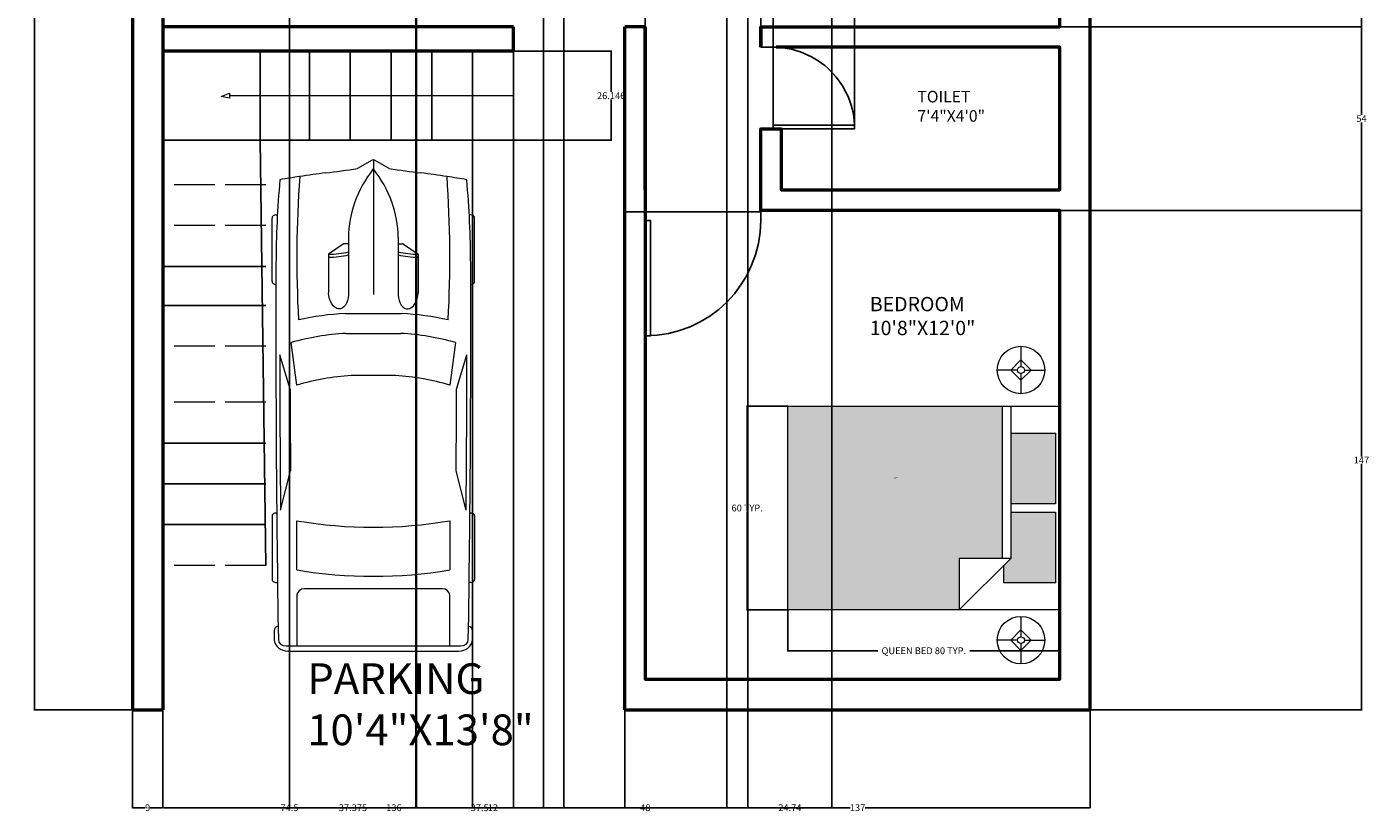
# Model space of a CAD drawing. Units: inches. Extents: x 32 to 429, y 30 to 648.
# Tile 1 of 3: x 32 to 427, y 30 to 261. Entities that reach past the tile are written whole.
import ezdxf

# ---------------------------------------------------------------- set-up
doc = ezdxf.new("R2010")
doc.units = ezdxf.units.IN
doc.header["$MEASUREMENT"] = 0
doc.linetypes.add('ACAD_ISO02W100', pattern=[15, 12, -3])
for name, color, linetype, lineweight in [('A-ANNO-DIMS', 2, 'Continuous', 18), ('A-ANNO-SYMB', 2, 'Continuous', 18), ('A-AREA-IDEN', 7, 'Continuous', 25), ('A-DOOR', 4, 'Continuous', 25), ('A-EQPM-VEHL', 8, 'Continuous', 18), ('A-FLOR-STRS', 7, 'Continuous', 25), ('A-FLOR-STRS-HIDN', 8, 'ACAD_ISO02W100', 18), ('A-FURN', 9, 'Continuous', 18), ('A-FURN-PATT', 252, 'Continuous', 13), ('A-WALL', 7, 'Continuous', 50)]:
    doc.layers.add(name, color=color, linetype=linetype, lineweight=lineweight)
doc.styles.get("Standard").update_dxf_attribs({"font": 'arial.ttf'})
doc.dimstyles.get("Standard").update_dxf_attribs({"dimtxt": 2, "dimasz": 0.18, "dimexe": 0.18, "dimexo": 0.0625, "dimgap": 0.09, "dimtad": 0, "dimtih": 1, "dimtoh": 1, "dimrnd": 2, "dimzin": 0, "dimdsep": 46, "dimlunit": 3, "dimtxsty": 'Standard', "dimcen": 0.09, "dimadec": 0, "dimazin": 0, "dimtfac": 1, "dimtofl": 0, "dimtmove": 0, "dimatfit": 3, "dimfxl": 1, "dimtolj": 1, "dimtzin": 0, "dimarcsym": 0})
pattern_1 = [(0, (0, -434.5), (0.03125, 0.0625), [0, -0.0625])]

# ---------------------------------------------------------------- blocks, each defined once
blk = doc.blocks.new('*U5')
for p, q in [((21.1, 37.41), (21.1, 36.83)), ((46.55, 38.89), (22.35, 38.89)), ((47.8, 37.39), (47.8, 37.41)), ((135.45, 37.07), (135.45, 37.41)), ((136.7, 38.89), (160.9, 38.89)), ((162.15, 37.41), (162.15, 36.77)), ((70.03, 31.54), (86.41, 29.35)), ((87.99, 31.87), (74.76, 35.92)), ((134.31, 35.6), (119.29, 31.78)), ((186.47, -33.5), (186.47, 33.5)), ((188.4, -32.76), (188.4, 32.76)), ((138.42, 29.35), (157.25, 29.35)), ((164.52, 26.39), (164.52, -26.39)), ((186.47, 29.35), (167.01, 29.35)), ((32.27, 11.63), (36.13, 17.17)), ((36.13, 17.17), (50.94, 17.17)), ((32.12, 9.51), (32.12, 11.15)), ((58.92, -10.77), (58.92, 10.77)), ((66.55, -10.53), (66.55, 10.53)), ((186.47, -10.53), (186.47, 10.53)), ((3.27, 6.13), (0.1, 0.41)), ((29.77, 9.51), (51.68, 9.51)), ((82.74, 8.5), (82.74, -8.5)), ((0, 0), (51.68, 0)), ((0.1, -0.41), (3.27, -6.13)), ((29.77, -9.51), (51.68, -9.51)), ((32.12, -9.51), (32.12, -11.15)), ((32.27, -11.63), (36.13, -17.17)), ((36.13, -17.17), (50.94, -17.17)), ((86.41, -29.35), (70.03, -31.54)), ((157.25, -29.35), (138.42, -29.35)), ((167.01, -29.35), (186.47, -29.35)), ((87.99, -31.87), (74.76, -35.92)), ((134.31, -35.6), (119.29, -31.78)), ((21.1, -37.41), (21.1, -36.83)), ((46.55, -38.89), (22.35, -38.89)), ((47.8, -37.39), (47.8, -37.41)), ((135.45, -37.07), (135.45, -37.41)), ((136.7, -38.89), (160.9, -38.89)), ((162.15, -37.41), (162.15, -36.77))]:
    blk.add_line(p, q)
for centre, major_axis, ratio, start_param, end_param in [((41.19, -490.86), (0, 528.23), 0.842304, 0.00281, 0.075598), ((22.35, 37.41), (0, -1.48), 0.842304, 3.141593, 4.712389), ((64.48, -10555.62), (0, 10593.03), 0.842304, -0.013397, 0.002797), ((46.55, 37.41), (0, 1.48), 0.842304, -1.570796, 0), ((136.7, 37.41), (0, -1.48), 0.842304, 3.141593, 4.712389), ((160.9, 37.41), (0, 1.48), 0.842304, -1.570796, 0), ((180.63, 35.84), (0, 2.22), 0.842304, -0.013017, 1.249894), ((64.48, -10556.36), (0, 10595.31), 0.842304, -0.013397, -0.013017), ((183.98, 33.5), (0, -2.96), 0.842304, 1.570796, 3.128196), ((183.98, 32.76), (0, -5.25), 0.842304, 1.570796, 3.128196), ((266.03, -27.52), (0, 313.31), 0.842304, 1.367076, 1.39176), ((135.29, 5.39), (0, 81.77), 0.842304, 1.245306, 1.50788), ((64.48, -10555.62), (0, -10591.55), 0.842304, 3.133765, 3.140441), ((95.79, -3666.35), (0, -3698.24), 0.842304, 3.134049, 3.144098), ((259.18, -27.52), (0, -305.3), 0.842304, 4.528606, 4.561838), ((37.47, -593.96), (0, -623.33), 0.842304, 3.096046, 3.200911), ((134.4, 5.39), (0, -89.78), 0.842304, 4.449482, 4.652344), ((149.6, 2.8), (0, -79.58), 0.842304, 4.372215, 4.640744), ((17.08, 0), (0, 147.02), 0.842304, 4.511394, 4.913384), ((35.91, 0), (0, 147.02), 0.842304, 4.511394, 4.913384), ((167.01, 26.39), (0, 2.96), 0.842304, 0, 1.570796), ((-204.49, 52.4), (0, -250.96), 0.842304, 1.385369, 1.434372), ((13.04, 17.01), (0, 27.42), 0.842304, 4.435146, 4.718221), ((14.2, 17.01), (0, 27.42), 0.842304, 4.435146, 4.718221), ((50.79, 13.34), (6.34, -0.36), 0.603834, -1.395552, 1.581315), ((32.75, 11.15), (0, 0.74), 0.842304, 0.879714, 1.570796), ((29.77, -46.66), (0, 56.17), 0.842304, 0, 0.590319), ((0.62, 0), (0, -0.74), 0.842304, 4.131459, 5.293319), ((29.77, 46.66), (0, 56.17), 0.842304, 2.551274, 3.141593), ((-204.49, -52.4), (0, 250.96), 0.842304, -1.434372, -1.385369), ((13.04, -17.01), (0, -27.42), 0.842304, 1.564964, 1.848039), ((14.2, -17.01), (0, -27.42), 0.842304, 1.564964, 1.848039), ((149.6, -2.8), (0, -79.58), 0.842304, -1.499151, -1.230623), ((32.75, -11.15), (0, -0.74), 0.842304, 4.712389, 5.403472), ((134.4, -5.39), (0, -89.78), 0.842304, -1.510751, -1.307889), ((135.29, -5.39), (0, -81.77), 0.842304, -1.50788, -1.245306), ((259.18, 27.52), (0, 305.3), 0.842304, 1.721348, 1.754579), ((266.03, 27.52), (0, 313.31), 0.842304, 1.749832, 1.774517), ((37.47, 593.96), (0, -623.33), 0.842304, -0.059319, 0.045547), ((167.01, -26.39), (0, -2.96), 0.842304, 4.712389, 6.283185), ((41.19, 490.86), (0, -528.23), 0.842304, -0.075598, -0.00281), ((64.48, 10555.62), (0, -10591.55), 0.842304, 0.001152, 0.007828), ((95.79, 3666.35), (0, -3698.24), 0.842304, -0.002505, 0.007544), ((183.98, -33.5), (0, 2.96), 0.842304, 3.15499, 4.712389), ((183.98, -32.76), (0, -5.25), 0.842304, 0.013397, 1.570796), ((22.35, -37.41), (0, 1.48), 0.842304, 1.570796, 3.141593), ((64.48, 10555.62), (0, 10593.03), 0.842304, 3.138796, 3.15499), ((46.55, -37.41), (0, -1.48), 0.842304, 0, 1.570796), ((136.7, -37.41), (0, -1.48), 0.842304, -1.570796, 0), ((160.9, -37.41), (0, 1.48), 0.842304, 3.141593, 4.712389), ((180.63, -35.84), (0, -2.22), 0.842304, -1.249894, 0.013017), ((64.48, 10556.36), (0, 10595.31), 0.842304, 3.15461, 3.15499)]:
    blk.add_ellipse(centre, major_axis=major_axis, ratio=ratio, start_param=start_param, end_param=end_param)
at = {"extrusion": (0, 0, -1)}
blk.add_ellipse((50.79, -13.34), major_axis=(6.34, 0.36), ratio=0.603834, start_param=-1.395552, end_param=1.581315, dxfattribs=at)
blk = doc.blocks.new('*U7')
for p, q in [((0, 0), (0, 6)), ((40, 0), (40, 6))]:
    blk.add_line(p, q)
blk.add_lwpolyline([(0, 0), (0, -40), (1.75, -40), (1.75, 0)], close=True)
blk.add_arc((0, 0), 40, 270, 0)
blk = doc.blocks.new('Bed - Queen')
for p, q in [((0, -80.00003), (0, 0)), ((0, 0), (59.99999, 0)), ((59.99999, 0), (59.99999, -80.00003)), ((7.99999, -1.2), (28.79998, -1.2)), ((7.99999, -14.4), (7.99999, -1.2)), ((28.79998, -1.2), (28.79998, -14.4)), ((31.19999, -1.2), (51.99999, -1.2)), ((31.19999, -14.4), (31.19999, -1.2)), ((51.99999, -1.2), (51.99999, -16.4)), ((0, -14.4), (44.8, -14.4)), ((59.99999, -29.6), (44.8, -14.4)), ((44.8, -14.4), (44.8, -29.6)), ((44.8, -16.8), (0, -16.8)), ((51.99999, -16.4), (46.79936, -16.4)), ((44.8, -29.6), (59.99999, -29.6)), ((59.99999, -80.00003), (0, -80.00003))]:
    blk.add_line(p, q)
blk = doc.blocks.new('Lamp - Table')
for p, q in [((0, 7), (0, 1)), ((-1, 0), (-7, 0)), ((0, 3), (-3, 0)), ((-3, 0), (0, -3)), ((3, 0), (0, 3)), ((0, -3), (3, 0)), ((1, 0), (7, 0)), ((0, -1), (0, -7))]:
    blk.add_line(p, q)
for radius in [7, 1]:
    blk.add_circle((0, 0), radius)
blk = doc.blocks.new('*D17')
at = {"layer": 'A-ANNO-DIMS', "color": 0, "lineweight": -2, "transparency": 16777216}
for p, q in [((256.39, 89.31), (256.39, 77.2)), ((336.39, 89.31), (336.39, 77.2)), ((256.57, 77.38), (282.82, 77.38)), ((336.21, 77.38), (309.97, 77.38))]:
    blk.add_line(p, q, dxfattribs=at)
at = {"layer": 'A-ANNO-DIMS', "color": 0, "transparency": 16777216}
for points in [[(256.57, 77.41), (256.57, 77.35), (256.39, 77.38)], [(336.21, 77.41), (336.21, 77.35), (336.39, 77.38)]]:
    blk.add_solid(points, dxfattribs=at)
at = {"layer": 'Defpoints', "color": 0, "transparency": 16777216}
for p in [(256.39, 89.38), (336.39, 89.38), (336.39, 77.38)]:
    blk.add_point(p, dxfattribs=at)
at = {"layer": 'A-ANNO-DIMS', "color": 0, "transparency": 16777216, "insert": (296.39, 77.38), "char_height": 2, "attachment_point": 5}
blk.add_mtext('\\A1;QUEEN BED 80 TYP.', dxfattribs=at)
blk = doc.blocks.new('*D18')
at = {"layer": 'A-ANNO-DIMS', "color": 0, "lineweight": -2, "transparency": 16777216}
for p, q in [((256.33, 149.38), (244.21, 149.38)), ((244.39, 149.2), (244.39, 120.49)), ((244.39, 89.56), (244.39, 118.27)), ((256.33, 89.38), (244.21, 89.38))]:
    blk.add_line(p, q, dxfattribs=at)
at = {"layer": 'A-ANNO-DIMS', "color": 0, "transparency": 16777216}
for points in [[(244.36, 149.2), (244.42, 149.2), (244.39, 149.38)], [(244.36, 89.56), (244.42, 89.56), (244.39, 89.38)]]:
    blk.add_solid(points, dxfattribs=at)
at = {"layer": 'Defpoints', "color": 0, "transparency": 16777216}
for p in [(256.39, 149.38), (244.39, 89.38), (256.39, 89.38)]:
    blk.add_point(p, dxfattribs=at)
at = {"layer": 'A-ANNO-DIMS', "color": 0, "transparency": 16777216, "insert": (244.39, 119.38), "char_height": 2, "attachment_point": 5}
blk.add_mtext('\\A1;60 TYP.', dxfattribs=at)
blk = doc.blocks.new('*D34')
at = {"layer": 'A-ANNO-DIMS', "color": 0, "lineweight": -2, "transparency": 16777216}
for p, q in [((63.33, 617.99), (34.41, 617.99)), ((34.59, 617.81), (34.59, 340.1)), ((34.59, 60.17), (34.59, 337.88)), ((63.33, 59.99), (34.41, 59.99))]:
    blk.add_line(p, q, dxfattribs=at)
at = {"layer": 'A-ANNO-DIMS', "color": 0, "transparency": 16777216}
for points in [[(34.56, 617.81), (34.62, 617.81), (34.59, 617.99)], [(34.56, 60.17), (34.62, 60.17), (34.59, 59.99)]]:
    blk.add_solid(points, dxfattribs=at)
at = {"layer": 'Defpoints', "color": 0, "transparency": 16777216}
for p in [(34.59, 617.99), (63.39, 617.99), (63.39, 59.99)]:
    blk.add_point(p, dxfattribs=at)
at = {"layer": 'A-ANNO-DIMS', "color": 0, "transparency": 16777216, "insert": (34.59, 338.99), "char_height": 2, "attachment_point": 5}
blk.add_mtext('\\A1;558', dxfattribs=at)
blk = doc.blocks.new('*D35')
at = {"layer": 'A-ANNO-DIMS', "color": 0, "lineweight": -2, "transparency": 16777216}
for p, q in [((63.39, 59.93), (63.39, 31.01)), ((72.39, 59.93), (72.39, 31.01)), ((63.57, 31.19), (67.15, 31.19)), ((72.21, 31.19), (68.64, 31.19))]:
    blk.add_line(p, q, dxfattribs=at)
at = {"layer": 'A-ANNO-DIMS', "color": 0, "transparency": 16777216}
for points in [[(63.57, 31.22), (63.57, 31.16), (63.39, 31.19)], [(72.21, 31.22), (72.21, 31.16), (72.39, 31.19)]]:
    blk.add_solid(points, dxfattribs=at)
at = {"layer": 'Defpoints', "color": 0, "transparency": 16777216}
for p in [(63.39, 59.99), (72.39, 59.99), (72.39, 31.19)]:
    blk.add_point(p, dxfattribs=at)
at = {"layer": 'A-ANNO-DIMS', "color": 0, "transparency": 16777216, "insert": (67.89, 31.19), "char_height": 2, "attachment_point": 5}
blk.add_mtext('\\A1;9', dxfattribs=at)
blk = doc.blocks.new('*D36')
at = {"layer": 'A-ANNO-DIMS', "color": 0, "lineweight": -2, "transparency": 16777216}
for p, q in [((72.39, 59.93), (72.39, 31.01)), ((208.39, 59.93), (208.39, 31.01)), ((72.57, 31.19), (138.19, 31.19)), ((208.21, 31.19), (142.6, 31.19))]:
    blk.add_line(p, q, dxfattribs=at)
at = {"layer": 'A-ANNO-DIMS', "color": 0, "transparency": 16777216}
for points in [[(72.57, 31.22), (72.57, 31.16), (72.39, 31.19)], [(208.21, 31.22), (208.21, 31.16), (208.39, 31.19)]]:
    blk.add_solid(points, dxfattribs=at)
at = {"layer": 'Defpoints', "color": 0, "transparency": 16777216}
for p in [(72.39, 59.99), (208.39, 59.99), (208.39, 31.19)]:
    blk.add_point(p, dxfattribs=at)
at = {"layer": 'A-ANNO-DIMS', "color": 0, "transparency": 16777216, "insert": (140.39, 31.19), "char_height": 2, "attachment_point": 5}
blk.add_mtext('\\A1;136', dxfattribs=at)
blk = doc.blocks.new('*D37')
at = {"layer": 'A-ANNO-DIMS', "color": 0, "lineweight": -2, "transparency": 16777216}
for p, q in [((208.39, 59.93), (208.39, 31.01)), ((345.39, 59.93), (345.39, 31.01)), ((208.57, 31.19), (274.69, 31.19)), ((345.21, 31.19), (279.1, 31.19))]:
    blk.add_line(p, q, dxfattribs=at)
at = {"layer": 'A-ANNO-DIMS', "color": 0, "transparency": 16777216}
for points in [[(208.57, 31.22), (208.57, 31.16), (208.39, 31.19)], [(345.21, 31.22), (345.21, 31.16), (345.39, 31.19)]]:
    blk.add_solid(points, dxfattribs=at)
at = {"layer": 'Defpoints', "color": 0, "transparency": 16777216}
for p in [(208.39, 59.99), (345.39, 59.99), (345.39, 31.19)]:
    blk.add_point(p, dxfattribs=at)
at = {"layer": 'A-ANNO-DIMS', "color": 0, "transparency": 16777216, "insert": (276.89, 31.19), "char_height": 2, "attachment_point": 5}
blk.add_mtext('\\A1;137', dxfattribs=at)
blk = doc.blocks.new('*D38')
at = {"layer": 'A-ANNO-DIMS', "color": 0, "lineweight": -2, "transparency": 16777216}
for p, q in [((336.46, 206.99), (425.41, 206.99)), ((425.23, 206.81), (425.23, 134.59)), ((425.23, 60.17), (425.23, 132.4)), ((345.46, 59.99), (425.41, 59.99))]:
    blk.add_line(p, q, dxfattribs=at)
at = {"layer": 'A-ANNO-DIMS', "color": 0, "transparency": 16777216}
for points in [[(425.2, 206.81), (425.26, 206.81), (425.23, 206.99)], [(425.2, 60.17), (425.26, 60.17), (425.23, 59.99)]]:
    blk.add_solid(points, dxfattribs=at)
at = {"layer": 'Defpoints', "color": 0, "transparency": 16777216}
for p in [(336.39, 206.99), (425.23, 206.99), (345.39, 59.99)]:
    blk.add_point(p, dxfattribs=at)
at = {"layer": 'A-ANNO-DIMS', "color": 0, "transparency": 16777216, "insert": (425.23, 133.49), "char_height": 2, "attachment_point": 5}
blk.add_mtext('\\A1;147', dxfattribs=at)
blk = doc.blocks.new('*D39')
at = {"layer": 'A-ANNO-DIMS', "color": 0, "lineweight": -2, "transparency": 16777216}
for p, q in [((336.46, 260.99), (425.41, 260.99)), ((425.23, 260.81), (425.23, 235.1)), ((425.23, 207.17), (425.23, 232.89)), ((336.46, 206.99), (425.41, 206.99))]:
    blk.add_line(p, q, dxfattribs=at)
at = {"layer": 'A-ANNO-DIMS', "color": 0, "transparency": 16777216}
for points in [[(425.2, 260.81), (425.26, 260.81), (425.23, 260.99)], [(425.2, 207.17), (425.26, 207.17), (425.23, 206.99)]]:
    blk.add_solid(points, dxfattribs=at)
at = {"layer": 'Defpoints', "color": 0, "transparency": 16777216}
for p in [(336.39, 260.99), (425.23, 260.99), (336.39, 206.99)]:
    blk.add_point(p, dxfattribs=at)
at = {"layer": 'A-ANNO-DIMS', "color": 0, "transparency": 16777216, "insert": (425.23, 233.99), "char_height": 2, "attachment_point": 5}
blk.add_mtext('\\A1;54', dxfattribs=at)
blk = doc.blocks.new('*D40')
at = {"layer": 'A-ANNO-DIMS', "color": 0, "lineweight": -2, "transparency": 16777216}
for p, q in [((336.46, 426.99), (425.41, 426.99)), ((425.23, 426.81), (425.23, 345.1)), ((425.23, 261.17), (425.23, 342.88)), ((336.46, 260.99), (425.41, 260.99))]:
    blk.add_line(p, q, dxfattribs=at)
at = {"layer": 'A-ANNO-DIMS', "color": 0, "transparency": 16777216}
for points in [[(425.2, 426.81), (425.26, 426.81), (425.23, 426.99)], [(425.2, 261.17), (425.26, 261.17), (425.23, 260.99)]]:
    blk.add_solid(points, dxfattribs=at)
at = {"layer": 'Defpoints', "color": 0, "transparency": 16777216}
for p in [(336.39, 426.99), (425.23, 426.99), (336.39, 260.99)]:
    blk.add_point(p, dxfattribs=at)
at = {"layer": 'A-ANNO-DIMS', "color": 0, "transparency": 16777216, "insert": (425.23, 343.99), "char_height": 2, "attachment_point": 5}
blk.add_mtext('\\A1;166', dxfattribs=at)
blk = doc.blocks.new('*D43')
at = {"layer": 'A-ANNO-DIMS', "color": 0, "lineweight": -2, "transparency": 16777216}
for p, q in [((72.39, 426.93), (72.39, 31.01)), ((146.89, 426.93), (146.89, 31.01)), ((72.57, 31.19), (106.96, 31.19)), ((146.71, 31.19), (112.33, 31.19))]:
    blk.add_line(p, q, dxfattribs=at)
at = {"layer": 'A-ANNO-DIMS', "color": 0, "transparency": 16777216}
for points in [[(72.57, 31.22), (72.57, 31.16), (72.39, 31.19)], [(146.71, 31.22), (146.71, 31.16), (146.89, 31.19)]]:
    blk.add_solid(points, dxfattribs=at)
at = {"layer": 'Defpoints', "color": 0, "transparency": 16777216}
for p in [(72.39, 426.99), (146.89, 426.99), (146.89, 31.19)]:
    blk.add_point(p, dxfattribs=at)
at = {"layer": 'A-ANNO-DIMS', "color": 0, "transparency": 16777216, "insert": (109.64, 31.19), "char_height": 2, "attachment_point": 5}
blk.add_mtext('\\A1;74.5', dxfattribs=at)
blk = doc.blocks.new('*D44')
at = {"layer": 'A-ANNO-DIMS', "color": 0, "lineweight": -2, "transparency": 16777216}
for p, q in [((146.89, 426.93), (146.89, 31.01)), ((184.39, 426.93), (184.39, 31.01)), ((147.07, 31.19), (162.95, 31.19)), ((184.21, 31.19), (168.34, 31.19))]:
    blk.add_line(p, q, dxfattribs=at)
at = {"layer": 'A-ANNO-DIMS', "color": 0, "transparency": 16777216}
for points in [[(147.07, 31.22), (147.07, 31.16), (146.89, 31.19)], [(184.21, 31.22), (184.21, 31.16), (184.39, 31.19)]]:
    blk.add_solid(points, dxfattribs=at)
at = {"layer": 'Defpoints', "color": 0, "transparency": 16777216}
for p in [(146.89, 426.99), (184.39, 426.99), (184.39, 31.19)]:
    blk.add_point(p, dxfattribs=at)
at = {"layer": 'A-ANNO-DIMS', "color": 0, "transparency": 16777216, "insert": (165.64, 31.19), "char_height": 2, "attachment_point": 5}
blk.add_mtext('\\A1;37.5', dxfattribs=at)
blk = doc.blocks.new('*D45')
at = {"layer": 'A-ANNO-DIMS', "color": 0, "lineweight": -2, "transparency": 16777216}
for p, q in [((190.39, 426.93), (190.39, 31.01)), ((238.39, 426.93), (238.39, 31.01)), ((190.57, 31.19), (212.83, 31.19)), ((238.21, 31.19), (215.96, 31.19))]:
    blk.add_line(p, q, dxfattribs=at)
at = {"layer": 'A-ANNO-DIMS', "color": 0, "transparency": 16777216}
for points in [[(190.57, 31.22), (190.57, 31.16), (190.39, 31.19)], [(238.21, 31.22), (238.21, 31.16), (238.39, 31.19)]]:
    blk.add_solid(points, dxfattribs=at)
at = {"layer": 'Defpoints', "color": 0, "transparency": 16777216}
for p in [(190.39, 426.99), (238.39, 426.99), (238.39, 31.19)]:
    blk.add_point(p, dxfattribs=at)
at = {"layer": 'A-ANNO-DIMS', "color": 0, "transparency": 16777216, "insert": (214.39, 31.19), "char_height": 2, "attachment_point": 5}
blk.add_mtext('\\A1;48', dxfattribs=at)
blk = doc.blocks.new('*D47')
at = {"layer": 'A-ANNO-DIMS', "color": 0, "lineweight": -2, "transparency": 16777216}
for p, q in [((214.39, 261.06), (214.39, 646.97)), ((214.57, 646.79), (229.88, 646.79)), ((248.21, 646.79), (232.91, 646.79)), ((248.39, 261.06), (248.39, 646.97))]:
    blk.add_line(p, q, dxfattribs=at)
at = {"layer": 'A-ANNO-DIMS', "color": 0, "transparency": 16777216}
for points in [[(214.57, 646.82), (214.57, 646.76), (214.39, 646.79)], [(248.21, 646.82), (248.21, 646.76), (248.39, 646.79)]]:
    blk.add_solid(points, dxfattribs=at)
at = {"layer": 'Defpoints', "color": 0, "transparency": 16777216}
for p in [(248.39, 646.79), (214.39, 260.99), (248.39, 260.99)]:
    blk.add_point(p, dxfattribs=at)
at = {"layer": 'A-ANNO-DIMS', "color": 0, "transparency": 16777216, "insert": (231.39, 646.79), "char_height": 2, "attachment_point": 5}
blk.add_mtext('\\A1;34', dxfattribs=at)
blk = doc.blocks.new('*D49')
at = {"layer": 'A-ANNO-DIMS', "color": 0, "lineweight": -2, "transparency": 16777216}
for p, q in [((109.64, 529.9), (109.64, 31.01)), ((147.02, 529.9), (147.02, 31.01)), ((109.82, 31.19), (124.08, 31.19)), ((146.84, 31.19), (132.58, 31.19))]:
    blk.add_line(p, q, dxfattribs=at)
at = {"layer": 'A-ANNO-DIMS', "color": 0, "transparency": 16777216}
for points in [[(109.82, 31.22), (109.82, 31.16), (109.64, 31.19)], [(146.84, 31.22), (146.84, 31.16), (147.02, 31.19)]]:
    blk.add_solid(points, dxfattribs=at)
at = {"layer": 'Defpoints', "color": 0, "transparency": 16777216}
for p in [(109.64, 529.96), (147.02, 529.96), (147.02, 31.19)]:
    blk.add_point(p, dxfattribs=at)
at = {"layer": 'A-ANNO-DIMS', "color": 0, "transparency": 16777216, "insert": (128.33, 31.19), "char_height": 2, "attachment_point": 5}
blk.add_mtext('\\A1;37.375', dxfattribs=at)
blk = doc.blocks.new('*D51')
at = {"layer": 'A-ANNO-DIMS', "color": 0, "lineweight": -2, "transparency": 16777216}
for p, q in [((244.58, 478.88), (244.58, 31.01)), ((269.32, 478.88), (269.32, 31.01)), ((244.76, 31.19), (253.47, 31.19)), ((269.14, 31.19), (260.43, 31.19))]:
    blk.add_line(p, q, dxfattribs=at)
at = {"layer": 'A-ANNO-DIMS', "color": 0, "transparency": 16777216}
for points in [[(244.76, 31.22), (244.76, 31.16), (244.58, 31.19)], [(269.14, 31.22), (269.14, 31.16), (269.32, 31.19)]]:
    blk.add_solid(points, dxfattribs=at)
at = {"layer": 'Defpoints', "color": 0, "transparency": 16777216}
for p in [(244.58, 478.95), (269.32, 478.95), (269.32, 31.19)]:
    blk.add_point(p, dxfattribs=at)
at = {"layer": 'A-ANNO-DIMS', "color": 0, "transparency": 16777216, "insert": (256.95, 31.19), "char_height": 2, "attachment_point": 5}
blk.add_mtext('\\A1;24.74', dxfattribs=at)
blk = doc.blocks.new('*D52')
at = {"layer": 'A-ANNO-DIMS', "color": 0, "lineweight": -2, "transparency": 16777216}
for p, q in [((252, 232.11), (252, 646.97)), ((252.18, 646.79), (260.54, 646.79)), ((275.84, 646.79), (267.48, 646.79)), ((276.02, 232.11), (276.02, 646.97))]:
    blk.add_line(p, q, dxfattribs=at)
at = {"layer": 'A-ANNO-DIMS', "color": 0, "transparency": 16777216}
for points in [[(252.18, 646.82), (252.18, 646.76), (252, 646.79)], [(275.84, 646.82), (275.84, 646.76), (276.02, 646.79)]]:
    blk.add_solid(points, dxfattribs=at)
at = {"layer": 'Defpoints', "color": 0, "transparency": 16777216}
for p in [(276.02, 646.79), (252, 232.04), (276.02, 232.04)]:
    blk.add_point(p, dxfattribs=at)
at = {"layer": 'A-ANNO-DIMS', "color": 0, "transparency": 16777216, "insert": (264.01, 646.79), "char_height": 2, "attachment_point": 5}
blk.add_mtext('\\A1;24.02', dxfattribs=at)
blk = doc.blocks.new('*D54')
at = {"layer": 'A-ANNO-DIMS', "color": 0, "lineweight": -2, "transparency": 16777216}
for p, q in [((163.55, 227.58), (163.55, 31.01)), ((175.55, 227.58), (175.55, 31.01)), ((163.73, 31.19), (168.13, 31.19)), ((175.37, 31.19), (170.96, 31.19))]:
    blk.add_line(p, q, dxfattribs=at)
at = {"layer": 'A-ANNO-DIMS', "color": 0, "transparency": 16777216}
for points in [[(163.73, 31.22), (163.73, 31.16), (163.55, 31.19)], [(175.37, 31.22), (175.37, 31.16), (175.55, 31.19)]]:
    blk.add_solid(points, dxfattribs=at)
at = {"layer": 'Defpoints', "color": 0, "transparency": 16777216}
for p in [(163.55, 227.65), (175.55, 227.65), (175.55, 31.19)]:
    blk.add_point(p, dxfattribs=at)
at = {"layer": 'A-ANNO-DIMS', "color": 0, "transparency": 16777216, "insert": (169.55, 31.19), "char_height": 2, "attachment_point": 5}
blk.add_mtext('\\A1;12', dxfattribs=at)
blk = doc.blocks.new('*D57')
at = {"layer": 'A-ANNO-DIMS', "color": 0, "lineweight": -2, "transparency": 16777216}
for p, q in [((175.61, 253.79), (204.53, 253.79)), ((204.35, 253.61), (204.35, 241.83)), ((204.35, 227.83), (204.35, 239.61)), ((175.61, 227.65), (204.53, 227.65))]:
    blk.add_line(p, q, dxfattribs=at)
at = {"layer": 'A-ANNO-DIMS', "color": 0, "transparency": 16777216}
for points in [[(204.32, 253.61), (204.38, 253.61), (204.35, 253.79)], [(204.32, 227.83), (204.38, 227.83), (204.35, 227.65)]]:
    blk.add_solid(points, dxfattribs=at)
at = {"layer": 'Defpoints', "color": 0, "transparency": 16777216}
for p in [(175.55, 253.79), (175.55, 227.65), (204.35, 227.65)]:
    blk.add_point(p, dxfattribs=at)
at = {"layer": 'A-ANNO-DIMS', "color": 0, "transparency": 16777216, "insert": (204.35, 240.72), "char_height": 2, "attachment_point": 5}
blk.add_mtext('\\A1;26.146', dxfattribs=at)

msp = doc.modelspace()

# ---------------------------------------------------------------- hatches: boundary and pattern name
at = {"layer": 'A-FURN-PATT'}
h = msp.add_hatch(dxfattribs=at)
h.set_pattern_fill('DOTS', color=256)
h.set_pattern_definition(pattern_1)
h.paths.add_polyline_path([(335.194, 141.3763), (321.994, 141.3763), (321.994, 120.5763), (335.194, 120.5763)])
h.paths.add_polyline_path([(335.194, 118.1763), (321.994, 118.1763), (321.994, 104.5763), (319.994, 102.5763), (319.994, 97.3763), (335.194, 97.3763)])
h.paths.add_polyline_path([(319.594, 149.3763), (256.3939, 149.3763), (256.3939, 89.3763), (306.794, 89.3763), (306.794, 104.5763), (319.594, 104.5763)])
h = msp.add_hatch(dxfattribs=at)
h.set_pattern_fill('DOTS', color=256)
h.set_pattern_definition(pattern_1)
h.paths.add_polyline_path([(319.594, 149.3763), (256.3939, 149.3763), (256.3939, 89.3763), (306.794, 89.3763), (306.794, 104.5763), (319.594, 104.5763)])

# ---------------------------------------------------------------- linework, layer by layer
at = {"layer": 'A-ANNO-SYMB'}
for p, q in [((89.5, 240.5), (92, 241.5)), ((92, 241.5), (92, 240.7197)), ((92, 240), (89.5, 240.5)), ((92, 241), (92, 241)), ((175.5464, 240.7197), (92, 240.7197)), ((92, 240.7197), (92, 240))]:
    msp.add_line(p, q, dxfattribs=at)
at = {"layer": 'A-DOOR'}
msp.add_line((248.3706, 206.589), (208.3942, 206.589), dxfattribs=at)
at = {"layer": 'A-FLOR-STRS'}
for p, q in [((115.5464, 253.7929), (115.5464, 227.6465)), ((127.5464, 253.7929), (127.5464, 227.6465)), ((139.5464, 253.7929), (139.5464, 227.6465)), ((151.5464, 253.7929), (151.5464, 227.6465)), ((163.5464, 253.7929), (163.5464, 227.6465)), ((175.5464, 253.7929), (175.5464, 227.6465)), ((175.5464, 227.6465), (72.3942, 227.6465)), ((101, 227.6465), (102.6949, 102.5)), ((102.6949, 190.5), (72.3942, 190.5)), ((102.6949, 179), (72.3942, 179)), ((102.6949, 179), (72.3942, 179)), ((102.6949, 138.5), (72.3942, 138.5)), ((102.6949, 126.5), (72.3942, 126.5)), ((102.6949, 114.5), (72.3942, 114.5))]:
    msp.add_line(p, q, dxfattribs=at)
msp.add_lwpolyline([(72.3942, 219.5), (72.3942, 253.7929), (101, 253.7929), (101, 227.6465)], dxfattribs=at)
at = {"layer": 'A-FLOR-STRS-HIDN'}
for p, q in [((102.6949, 214.5), (72.3942, 214.5)), ((102.6949, 202.5), (72.3942, 202.5)), ((102.6949, 190.5), (72.3942, 190.5)), ((102.6949, 179), (72.3942, 179)), ((102.6949, 167), (72.3942, 167)), ((102.6949, 150.5), (72.3942, 150.5)), ((102.6949, 138.5), (72.3942, 138.5)), ((102.6949, 126.5), (72.3942, 126.5)), ((102.6949, 114.5), (72.3942, 114.5)), ((102.6949, 102.5), (72.3942, 102.5))]:
    msp.add_line(p, q, dxfattribs=at)
at = {"layer": 'A-WALL'}
for p, q in [((175.5464, 260.9929), (72.3942, 260.9929)), ((175.5464, 253.7929), (175.5464, 260.9929)), ((214.3942, 260.9929), (208.3942, 260.9929)), ((208.3942, 212.9929), (208.3942, 260.9929)), ((214.3942, 212.9929), (214.3942, 260.9929)), ((248.3942, 260.9929), (248.3942, 254.9929)), ((175.5464, 253.7929), (72.3942, 253.7929))]:
    msp.add_line(p, q, dxfattribs=at)
for points in [[(208.3942, 59.9929), (345.3942, 59.9929), (345.3942, 617.9929), (63.3942, 617.9929), (63.3942, 59.9929)], [(248.394, 254.9928), (248.394, 260.9928), (336.394, 260.9928), (336.394, 608.9928), (72.394, 608.9928), (72.394, 59.9928)], [(208.3942, 59.9929), (208.3942, 260.9929)], [(214.3942, 260.9929), (214.3942, 68.9929), (336.3942, 68.9929), (336.3942, 196.9929)], [(214.3942, 68.9929), (336.3942, 68.9929), (336.3942, 206.9929), (248.3942, 206.9929), (248.3942, 230.9929), (254.3942, 230.9929), (254.3942, 212.9929), (336.3942, 212.9929), (336.3942, 254.9929), (252.9424, 254.9929)], [(63.3942, 59.9929), (72.3942, 59.9929)]]:
    msp.add_lwpolyline(points, dxfattribs=at)

# ---------------------------------------------------------------- block references
at = {"layer": 'A-DOOR', "xscale": 0.6004652585317019, "yscale": 0.6004652585317019, "zscale": 0.6004652585317019, "rotation": 90.00000000000018}
msp.add_blockref('*U7', (251.997, 230.9929), dxfattribs=at)
at = {"layer": 'A-DOOR', "xscale": 0.8494094044284386, "yscale": 0.8494094044284386, "zscale": 0.8494094044284386}
msp.add_blockref('*U7', (214.3942, 204.0408), dxfattribs=at)
at = {"layer": 'A-EQPM-VEHL', "xscale": 0.7670724168358353, "yscale": 0.7670724168358353, "zscale": 0.7670724168358353, "rotation": 270}
msp.add_blockref('*U5', (134.3295, 221.8177), dxfattribs=at)
at = {"layer": 'A-FURN'}
for p in [(325, 160), (325, 80.5)]:
    msp.add_blockref('Lamp - Table', p, dxfattribs=at)
at = {"layer": 'A-FURN', "rotation": 270}
msp.add_blockref('Bed - Queen', (336.394, 149.3763), dxfattribs=at)

# ---------------------------------------------------------------- texts
at = {"layer": 'A-AREA-IDEN', "attachment_point": 1}
for s, width, gutter_width, insert, char_height in [('TOILET\\P7\'4"X4\'0"', 8.502953, 17.0059, (294.497, 242.1609), 3.40118), ('BEDROOM\\P10\'8"X12\'0"', 38.275318, 19.1377, (280.5, 181.5), 4.210285)]:
    msp.add_mtext_dynamic_manual_height_columns(s, width=width, gutter_width=gutter_width, heights=[0], dxfattribs=dict(at, insert=insert, char_height=char_height))
for s, insert, char_height in [('"X12\'0BEDROOM\\P10\'8"', (287.5, 128.5), 0.2), ('PARKING\\P10\'4"X13\'8"', (114.8919, 73.6828), 9.03471)]:
    msp.add_mtext(s, dxfattribs=dict(at, insert=insert, char_height=char_height))

# ---------------------------------------------------------------- dimensions: what is measured, and where the dimension line sits
at = {"layer": 'A-ANNO-DIMS'}
for base, p1, p2, override, picture, middle in [((248.394, 646.7929), (214.3942, 260.9929), (248.394, 260.9928), {"dimdec": 0, "dimlfac": 1, "dimrnd": 0, "dimzin": 0, "dimdsep": 46, "dimlunit": 2}, '*D47', (231.3941, 646.7929)), ((276.0156, 646.7929), (251.997, 232.0437), (276.0156, 232.0437), {"dimdec": 2, "dimlfac": 1, "dimrnd": 0, "dimzin": 0, "dimdsep": 46, "dimlunit": 2}, '*D52', (264.0063, 646.7929)), ((147.0192, 31.1928), (109.6441, 529.9584), (147.0192, 529.9584), {"dimdec": 3, "dimlfac": 1, "dimrnd": 0, "dimzin": 0, "dimdsep": 46, "dimlunit": 2}, '*D49', (128.3316, 31.1928)), ((269.3206, 31.1928), (244.5793, 478.9469), (269.3206, 478.9469), {"dimdec": 2, "dimlfac": 1, "dimrnd": 0, "dimzin": 0, "dimdsep": 46, "dimlunit": 2}, '*D51', (256.95, 31.1928)), ((146.8939, 31.1928), (72.3942, 426.9929), (146.8939, 426.9929), {"dimdec": 1, "dimlfac": 1, "dimrnd": 0, "dimzin": 0, "dimdsep": 46, "dimlunit": 2}, '*D43', (109.6441, 31.1928)), ((184.3942, 31.1928), (146.8939, 426.9929), (184.3942, 426.9929), {"dimdec": 1, "dimlfac": 1, "dimrnd": 0, "dimzin": 0, "dimdsep": 46, "dimlunit": 2}, '*D44', (165.6441, 31.1928)), ((238.3942, 31.1928), (190.3942, 426.9929), (238.3942, 426.9929), {"dimdec": 0, "dimlfac": 1, "dimrnd": 0, "dimzin": 0, "dimdsep": 46, "dimlunit": 2}, '*D45', (214.3942, 31.1928)), ((175.5464, 31.1928), (163.5464, 227.6465), (175.5464, 227.6465), {"dimdec": 0, "dimlfac": 1, "dimrnd": 0, "dimzin": 0, "dimdsep": 46, "dimlunit": 2}, '*D54', (169.5464, 31.1928)), ((72.394, 31.1928), (63.3942, 59.9929), (72.394, 59.9928), {"dimdec": 0, "dimlfac": 1, "dimrnd": 0, "dimzin": 0, "dimdsep": 46, "dimlunit": 2}, '*D35', (67.8941, 31.1928)), ((208.3942, 31.1928), (72.394, 59.9928), (208.3942, 59.9929), {"dimdec": 0, "dimlfac": 1, "dimrnd": 0, "dimzin": 0, "dimdsep": 46, "dimlunit": 2}, '*D36', (140.3941, 31.1928)), ((345.3942, 31.1928), (208.3942, 59.9929), (345.3942, 59.9929), {"dimdec": 0, "dimlfac": 1, "dimrnd": 0, "dimzin": 0, "dimdsep": 46, "dimlunit": 2}, '*D37', (276.8942, 31.1928))]:
    dim = msp.add_linear_dim(base=base, p1=p1, p2=p2, dimstyle='Standard', override=override, dxfattribs=at)
    dim.commit()
    dim.dimension.update_dxf_attribs({"geometry": picture, "text_midpoint": middle})
for base, p1, p2, angle, override, picture, middle in [((34.5942, 617.9929), (63.3942, 59.9929), (63.3942, 617.9929), 90, {"dimdec": 0, "dimlfac": 1, "dimrnd": 0, "dimzin": 0, "dimdsep": 46, "dimlunit": 2}, '*D34', (34.5942, 338.9929)), ((425.2284, 426.9929), (336.394, 260.9928), (336.3942, 426.9929), 90, {"dimdec": 0, "dimlfac": 1, "dimrnd": 0, "dimzin": 0, "dimdsep": 46, "dimlunit": 2}, '*D40', (425.2284, 343.9929)), ((425.2284, 260.9928), (336.3942, 206.9929), (336.394, 260.9928), 90, {"dimdec": 0, "dimlfac": 1, "dimrnd": 0, "dimzin": 0, "dimdsep": 46, "dimlunit": 2}, '*D39', (425.2284, 233.9929)), ((204.3464, 227.6465), (175.5464, 253.7929), (175.5464, 227.6465), 270, {"dimdec": 3, "dimlfac": 1, "dimrnd": 0, "dimzin": 0, "dimdsep": 46, "dimlunit": 2}, '*D57', (204.3464, 240.7197)), ((425.2284, 206.9929), (345.3942, 59.9929), (336.3942, 206.9929), 90, {"dimdec": 0, "dimlfac": 1, "dimrnd": 0, "dimzin": 0, "dimdsep": 46, "dimlunit": 2}, '*D38', (425.2284, 133.4929))]:
    dim = msp.add_linear_dim(base=base, p1=p1, p2=p2, angle=angle, dimstyle='Standard', override=override, dxfattribs=at)
    dim.commit()
    dim.dimension.update_dxf_attribs({"geometry": picture, "text_midpoint": middle})
dim = msp.add_linear_dim(base=(244.3939, 89.3763), p1=(256.3939, 149.3763), p2=(256.3939, 89.3763), angle=270, text='<> TYP.', dimstyle='Standard', override={"dimdec": 0, "dimlfac": 1, "dimrnd": 0, "dimzin": 0, "dimdsep": 46, "dimlunit": 2}, dxfattribs=at)
dim.commit()
dim.dimension.update_dxf_attribs({"geometry": '*D18', "text_midpoint": (244.3939, 119.3763)})
dim = msp.add_linear_dim(base=(336.394, 77.3763), p1=(256.3939, 89.3763), p2=(336.394, 89.3763), text='QUEEN BED <> TYP.', dimstyle='Standard', override={"dimdec": 0, "dimlfac": 1, "dimrnd": 0, "dimzin": 0, "dimdsep": 46, "dimlunit": 2}, dxfattribs=at)
dim.commit()
dim.dimension.update_dxf_attribs({"geometry": '*D17', "text_midpoint": (296.394, 77.3763)})

doc.saveas('drawing.dxf')
